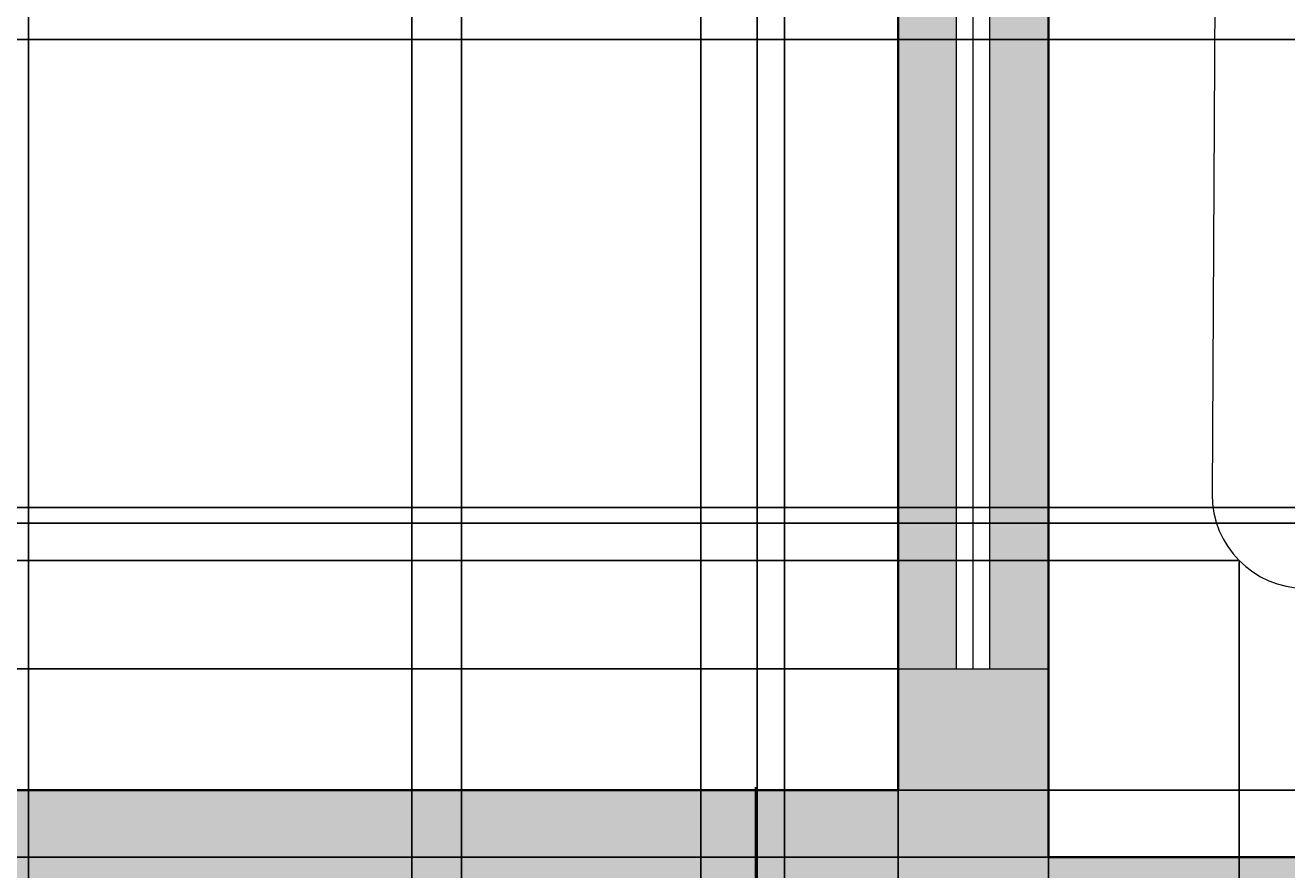
# Model space of a CAD drawing. Units: inches. Extents: x 818 to 1898, y 976 to 2364.
# Tile 29 of 96: x 1207 to 1282, y 1695 to 1746. Entities that reach past the tile are written whole.
import ezdxf

# ---------------------------------------------------------------- set-up
doc = ezdxf.new("R2010")
doc.units = ezdxf.units.IN
doc.header["$LTSCALE"] = 5
doc.header["$MEASUREMENT"] = 0
for name, color, linetype, lineweight in [('A-ANNO-DIMS', 2, 'Continuous', 18), ('A-FURN', 8, 'Continuous', 18), ('A-GLAZ', 4, 'Continuous', 18), ('A-WALL', 7, 'Continuous', 40)]:
    doc.layers.add(name, color=color, linetype=linetype, lineweight=lineweight)
doc.layers.add('A-GLAZ-PATT', color=141, linetype='Continuous', lineweight=9, true_color=0xadddf7)
doc.layers.add('A-WALL-PATT', color=251, linetype='Continuous', lineweight=13, true_color=0x636466)
doc.styles.get("Standard").update_dxf_attribs({"font": 'arial.ttf'})
doc.dimstyles.get("Standard").update_dxf_attribs({"dimtxt": 0.18, "dimasz": 0.18, "dimexe": 0.18, "dimexo": 0.0625, "dimgap": 0.09, "dimtad": 0, "dimtih": 1, "dimtoh": 1, "dimdec": 4, "dimzin": 0, "dimdsep": 46, "dimtxsty": 'Standard', "dimcen": 0.09, "dimadec": 0, "dimazin": 0, "dimtfac": 1, "dimtdec": 4, "dimtofl": 0, "dimtmove": 0, "dimatfit": 3, "dimfxl": 1, "dimtolj": 1, "dimtzin": 0, "dimarcsym": 0})

# ---------------------------------------------------------------- blocks, each defined once
blk = doc.blocks.new('SOFA-3-SEAT')
blk.add_line((39.87, 35.861), (5.697, 36.046))
blk.add_arc((5.667, 30.46), 5.586, 89.68982, 179.68982)
blk = doc.blocks.new('*D42')
at = {"layer": 'A-ANNO-DIMS', "color": 0, "lineweight": -2, "ltscale": 5, "transparency": 16777216}
for p, q in [((1250.195, 1683.07), (1250.195, 1700.259)), ((1250.375, 1700.079), (1306.123, 1700.079)), ((1363.82, 1700.079), (1308.072, 1700.079)), ((1364, 1683.07), (1364, 1700.259))]:
    blk.add_line(p, q, dxfattribs=at)
at = {"layer": 'A-ANNO-DIMS', "color": 0, "ltscale": 5, "transparency": 16777216}
for points in [[(1250.375, 1700.109), (1250.375, 1700.049), (1250.195, 1700.079)], [(1363.82, 1700.109), (1363.82, 1700.049), (1364, 1700.079)]]:
    blk.add_solid(points, dxfattribs=at)
at = {"layer": 'Defpoints', "color": 0, "ltscale": 5, "transparency": 16777216}
for p in [(1364, 1700.079), (1250.195, 1683.008), (1364, 1683.008)]:
    blk.add_point(p, dxfattribs=at)
at = {"layer": 'A-ANNO-DIMS', "color": 0, "ltscale": 5, "transparency": 16777216, "insert": (1307.097, 1700.079), "char_height": 0.18, "attachment_point": 5}
blk.add_mtext('\\A1;SOFA 114 TYP.', dxfattribs=at)
blk = doc.blocks.new('*D59')
at = {"layer": 'A-ANNO-DIMS', "color": 0, "lineweight": -2, "ltscale": 5, "transparency": 16777216}
for p, q in [((1251.643, 2300.393), (818.026, 2300.393)), ((818.206, 2300.213), (818.206, 1669.95)), ((818.206, 1039.323), (818.206, 1669.586)), ((896.051, 1039.143), (818.026, 1039.143))]:
    blk.add_line(p, q, dxfattribs=at)
at = {"layer": 'A-ANNO-DIMS', "color": 0, "ltscale": 5, "transparency": 16777216}
for points in [[(818.176, 2300.213), (818.236, 2300.213), (818.206, 2300.393)], [(818.176, 1039.323), (818.236, 1039.323), (818.206, 1039.143)]]:
    blk.add_solid(points, dxfattribs=at)
at = {"layer": 'Defpoints', "color": 0, "ltscale": 5, "transparency": 16777216}
for p in [(818.206, 2300.393), (1251.706, 2300.393), (896.114, 1039.143)]:
    blk.add_point(p, dxfattribs=at)
at = {"layer": 'A-ANNO-DIMS', "color": 0, "ltscale": 5, "transparency": 16777216, "insert": (818.206, 1669.768), "char_height": 0.18, "attachment_point": 5}
blk.add_mtext('\\A1;1261.2', dxfattribs=at)
blk = doc.blocks.new('*D61')
at = {"layer": 'A-ANNO-DIMS', "color": 0, "lineweight": -2, "ltscale": 5, "transparency": 16777216}
for p, q in [((1071.725, 1203.027), (1071.725, 2363.873)), ((1430.725, 1203.027), (1430.725, 2363.873)), ((1071.905, 2363.693), (1250.936, 2363.693)), ((1430.545, 2363.693), (1251.514, 2363.693))]:
    blk.add_line(p, q, dxfattribs=at)
at = {"layer": 'A-ANNO-DIMS', "color": 0, "ltscale": 5, "transparency": 16777216}
for points in [[(1071.905, 2363.723), (1071.905, 2363.663), (1071.725, 2363.693)], [(1430.545, 2363.723), (1430.545, 2363.663), (1430.725, 2363.693)]]:
    blk.add_solid(points, dxfattribs=at)
at = {"layer": 'Defpoints', "color": 0, "ltscale": 5, "transparency": 16777216}
for p in [(1430.725, 2363.693), (1071.725, 1202.964), (1430.725, 1202.964)]:
    blk.add_point(p, dxfattribs=at)
at = {"layer": 'A-ANNO-DIMS', "color": 0, "ltscale": 5, "transparency": 16777216, "insert": (1251.225, 2363.693), "char_height": 0.18, "attachment_point": 5}
blk.add_mtext('\\A1;359', dxfattribs=at)
blk = doc.blocks.new('*D64')
at = {"layer": 'A-ANNO-DIMS', "color": 0, "lineweight": -2, "ltscale": 5, "transparency": 16777216}
for p, q in [((1197.725, 1501.141), (1197.725, 2363.873)), ((1430.725, 1501.141), (1430.725, 2363.873)), ((1197.905, 2363.693), (1313.935, 2363.693)), ((1430.545, 2363.693), (1314.516, 2363.693))]:
    blk.add_line(p, q, dxfattribs=at)
at = {"layer": 'A-ANNO-DIMS', "color": 0, "ltscale": 5, "transparency": 16777216}
for points in [[(1197.905, 2363.723), (1197.905, 2363.663), (1197.725, 2363.693)], [(1430.545, 2363.723), (1430.545, 2363.663), (1430.725, 2363.693)]]:
    blk.add_solid(points, dxfattribs=at)
at = {"layer": 'Defpoints', "color": 0, "ltscale": 5, "transparency": 16777216}
for p in [(1430.725, 2363.693), (1197.725, 1501.078), (1430.725, 1501.078)]:
    blk.add_point(p, dxfattribs=at)
at = {"layer": 'A-ANNO-DIMS', "color": 0, "ltscale": 5, "transparency": 16777216, "insert": (1314.225, 2363.693), "char_height": 0.18, "attachment_point": 5}
blk.add_mtext('\\A1;233', dxfattribs=at)
blk = doc.blocks.new('*D83')
at = {"layer": 'A-ANNO-DIMS', "color": 0, "lineweight": -2, "ltscale": 5, "transparency": 16777216}
for p, q in [((1197.725, 1700.141), (1197.725, 2363.873)), ((1258.725, 1700.141), (1258.725, 2363.873)), ((1197.905, 2363.693), (1228.023, 2363.693)), ((1258.545, 2363.693), (1228.427, 2363.693))]:
    blk.add_line(p, q, dxfattribs=at)
at = {"layer": 'A-ANNO-DIMS', "color": 0, "ltscale": 5, "transparency": 16777216}
for points in [[(1197.905, 2363.723), (1197.905, 2363.663), (1197.725, 2363.693)], [(1258.545, 2363.723), (1258.545, 2363.663), (1258.725, 2363.693)]]:
    blk.add_solid(points, dxfattribs=at)
at = {"layer": 'Defpoints', "color": 0, "ltscale": 5, "transparency": 16777216}
for p in [(1258.725, 2363.693), (1197.725, 1700.078), (1258.725, 1700.078)]:
    blk.add_point(p, dxfattribs=at)
at = {"layer": 'A-ANNO-DIMS', "color": 0, "ltscale": 5, "transparency": 16777216, "insert": (1228.225, 2363.693), "char_height": 0.18, "attachment_point": 5}
blk.add_mtext('\\A1;61', dxfattribs=at)
blk = doc.blocks.new('*D85')
at = {"layer": 'A-ANNO-DIMS', "color": 0, "lineweight": -2, "ltscale": 5, "transparency": 16777216}
for p, q in [((1258.788, 2053.078), (1897.916, 2053.078)), ((1897.736, 2052.898), (1897.736, 1876.76)), ((1897.736, 1700.258), (1897.736, 1876.396)), ((1258.788, 1700.078), (1897.916, 1700.078))]:
    blk.add_line(p, q, dxfattribs=at)
at = {"layer": 'A-ANNO-DIMS', "color": 0, "ltscale": 5, "transparency": 16777216}
for points in [[(1897.706, 2052.898), (1897.766, 2052.898), (1897.736, 2053.078)], [(1897.706, 1700.258), (1897.766, 1700.258), (1897.736, 1700.078)]]:
    blk.add_solid(points, dxfattribs=at)
at = {"layer": 'Defpoints', "color": 0, "ltscale": 5, "transparency": 16777216}
for p in [(1258.725, 2053.078), (1897.736, 2053.078), (1258.725, 1700.078)]:
    blk.add_point(p, dxfattribs=at)
at = {"layer": 'A-ANNO-DIMS', "color": 0, "ltscale": 5, "transparency": 16777216, "insert": (1897.736, 1876.578), "char_height": 0.18, "attachment_point": 5}
blk.add_mtext('\\A1;353', dxfattribs=at)
blk = doc.blocks.new('*D95')
at = {"layer": 'A-ANNO-DIMS', "color": 0, "lineweight": -2, "ltscale": 5, "transparency": 16777216}
for p, q in [((1173.542, 1071.118), (1173.542, 2363.873)), ((1229.647, 1071.118), (1229.647, 2363.873)), ((1173.722, 2363.693), (1201.288, 2363.693)), ((1229.467, 2363.693), (1201.901, 2363.693))]:
    blk.add_line(p, q, dxfattribs=at)
at = {"layer": 'A-ANNO-DIMS', "color": 0, "ltscale": 5, "transparency": 16777216}
for points in [[(1173.722, 2363.723), (1173.722, 2363.663), (1173.542, 2363.693)], [(1229.467, 2363.723), (1229.467, 2363.663), (1229.647, 2363.693)]]:
    blk.add_solid(points, dxfattribs=at)
at = {"layer": 'Defpoints', "color": 0, "ltscale": 5, "transparency": 16777216}
for p in [(1229.647, 2363.693), (1173.542, 1071.055), (1229.647, 1071.055)]:
    blk.add_point(p, dxfattribs=at)
at = {"layer": 'A-ANNO-DIMS', "color": 0, "ltscale": 5, "transparency": 16777216, "insert": (1201.595, 2363.693), "char_height": 0.18, "attachment_point": 5}
blk.add_mtext('\\A1;56.1', dxfattribs=at)
blk = doc.blocks.new('*D96')
at = {"layer": 'A-ANNO-DIMS', "color": 0, "lineweight": -2, "ltscale": 5, "transparency": 16777216}
for p, q in [((1229.647, 1071.118), (1229.647, 2363.873)), ((1284.17, 1071.118), (1284.17, 2363.873)), ((1229.827, 2363.693), (1256.516, 2363.693)), ((1283.99, 2363.693), (1257.301, 2363.693))]:
    blk.add_line(p, q, dxfattribs=at)
at = {"layer": 'A-ANNO-DIMS', "color": 0, "ltscale": 5, "transparency": 16777216}
for points in [[(1229.827, 2363.723), (1229.827, 2363.663), (1229.647, 2363.693)], [(1283.99, 2363.723), (1283.99, 2363.663), (1284.17, 2363.693)]]:
    blk.add_solid(points, dxfattribs=at)
at = {"layer": 'Defpoints', "color": 0, "ltscale": 5, "transparency": 16777216}
for p in [(1284.17, 2363.693), (1229.647, 1071.055), (1284.17, 1071.055)]:
    blk.add_point(p, dxfattribs=at)
at = {"layer": 'A-ANNO-DIMS', "color": 0, "ltscale": 5, "transparency": 16777216, "insert": (1256.909, 2363.693), "char_height": 0.18, "attachment_point": 5}
blk.add_mtext('\\A1;54.52', dxfattribs=at)
blk = doc.blocks.new('*D119')
at = {"layer": 'A-ANNO-DIMS', "color": 0, "lineweight": -2, "ltscale": 5, "transparency": 16777216}
for p, q in [((1766.29, 1716.987), (818.026, 1716.987)), ((818.206, 1716.807), (818.206, 1672.428)), ((818.206, 1627.685), (818.206, 1672.064)), ((1766.29, 1627.505), (818.026, 1627.505))]:
    blk.add_line(p, q, dxfattribs=at)
at = {"layer": 'A-ANNO-DIMS', "color": 0, "ltscale": 5, "transparency": 16777216}
for points in [[(818.176, 1716.807), (818.236, 1716.807), (818.206, 1716.987)], [(818.176, 1627.685), (818.236, 1627.685), (818.206, 1627.505)]]:
    blk.add_solid(points, dxfattribs=at)
at = {"layer": 'Defpoints', "color": 0, "ltscale": 5, "transparency": 16777216}
for p in [(818.206, 1716.987), (1766.352, 1716.987), (1766.352, 1627.505)]:
    blk.add_point(p, dxfattribs=at)
at = {"layer": 'A-ANNO-DIMS', "color": 0, "ltscale": 5, "transparency": 16777216, "insert": (818.206, 1672.246), "char_height": 0.18, "attachment_point": 5}
blk.add_mtext('\\A1;89.48', dxfattribs=at)
blk = doc.blocks.new('*D120')
at = {"layer": 'A-ANNO-DIMS', "color": 0, "lineweight": -2, "ltscale": 5, "transparency": 16777216}
for p, q in [((1766.29, 1797.717), (818.026, 1797.717)), ((818.206, 1797.537), (818.206, 1757.534)), ((818.206, 1717.167), (818.206, 1757.17)), ((1766.29, 1716.987), (818.026, 1716.987))]:
    blk.add_line(p, q, dxfattribs=at)
at = {"layer": 'A-ANNO-DIMS', "color": 0, "ltscale": 5, "transparency": 16777216}
for points in [[(818.176, 1797.537), (818.236, 1797.537), (818.206, 1797.717)], [(818.176, 1717.167), (818.236, 1717.167), (818.206, 1716.987)]]:
    blk.add_solid(points, dxfattribs=at)
at = {"layer": 'Defpoints', "color": 0, "ltscale": 5, "transparency": 16777216}
for p in [(818.206, 1797.717), (1766.352, 1797.717), (1766.352, 1716.987)]:
    blk.add_point(p, dxfattribs=at)
at = {"layer": 'A-ANNO-DIMS', "color": 0, "ltscale": 5, "transparency": 16777216, "insert": (818.206, 1757.352), "char_height": 0.18, "attachment_point": 5}
blk.add_mtext('\\A1;80.73', dxfattribs=at)
blk = doc.blocks.new('*D145')
at = {"layer": 'A-ANNO-DIMS', "color": 0, "lineweight": -2, "ltscale": 5, "transparency": 16777216}
for p, q in [((1197.393, 2122.314), (1197.393, 975.663)), ((1232.609, 2122.314), (1232.609, 975.663)), ((1197.573, 975.843), (1214.608, 975.843)), ((1232.429, 975.843), (1215.394, 975.843))]:
    blk.add_line(p, q, dxfattribs=at)
at = {"layer": 'A-ANNO-DIMS', "color": 0, "ltscale": 5, "transparency": 16777216}
for points in [[(1197.573, 975.873), (1197.573, 975.813), (1197.393, 975.843)], [(1232.429, 975.873), (1232.429, 975.813), (1232.609, 975.843)]]:
    blk.add_solid(points, dxfattribs=at)
at = {"layer": 'Defpoints', "color": 0, "ltscale": 5, "transparency": 16777216}
for p in [(1197.393, 2122.377), (1232.609, 2122.377), (1232.609, 975.843)]:
    blk.add_point(p, dxfattribs=at)
at = {"layer": 'A-ANNO-DIMS', "color": 0, "ltscale": 5, "transparency": 16777216, "insert": (1215.001, 975.843), "char_height": 0.18, "attachment_point": 5}
blk.add_mtext('\\A1;35.22', dxfattribs=at)
blk = doc.blocks.new('*D215')
at = {"layer": 'A-ANNO-DIMS', "color": 0, "lineweight": -2, "ltscale": 5, "transparency": 16777216}
for p, q in [((1590.663, 1876.078), (818.026, 1876.078)), ((818.206, 1875.898), (818.206, 1781.76)), ((818.206, 1687.258), (818.206, 1781.396)), ((1511.663, 1687.078), (818.026, 1687.078))]:
    blk.add_line(p, q, dxfattribs=at)
at = {"layer": 'A-ANNO-DIMS', "color": 0, "ltscale": 5, "transparency": 16777216}
for points in [[(818.176, 1875.898), (818.236, 1875.898), (818.206, 1876.078)], [(818.176, 1687.258), (818.236, 1687.258), (818.206, 1687.078)]]:
    blk.add_solid(points, dxfattribs=at)
at = {"layer": 'Defpoints', "color": 0, "ltscale": 5, "transparency": 16777216}
for p in [(818.206, 1876.078), (1590.725, 1876.078), (1511.725, 1687.078)]:
    blk.add_point(p, dxfattribs=at)
at = {"layer": 'A-ANNO-DIMS', "color": 0, "ltscale": 5, "transparency": 16777216, "insert": (818.206, 1781.578), "char_height": 0.18, "attachment_point": 5}
blk.add_mtext('\\A1;189', dxfattribs=at)
blk = doc.blocks.new('*D222')
at = {"layer": 'A-ANNO-DIMS', "color": 0, "lineweight": -2, "ltscale": 5, "transparency": 16777216}
for p, q in [((1511.663, 1744.971), (818.026, 1744.971)), ((818.206, 1744.791), (818.206, 1730.69)), ((818.206, 1716.225), (818.206, 1730.327)), ((1511.663, 1716.045), (818.026, 1716.045))]:
    blk.add_line(p, q, dxfattribs=at)
at = {"layer": 'A-ANNO-DIMS', "color": 0, "ltscale": 5, "transparency": 16777216}
for points in [[(818.176, 1744.791), (818.236, 1744.791), (818.206, 1744.971)], [(818.176, 1716.225), (818.236, 1716.225), (818.206, 1716.045)]]:
    blk.add_solid(points, dxfattribs=at)
at = {"layer": 'Defpoints', "color": 0, "ltscale": 5, "transparency": 16777216}
for p in [(818.206, 1744.971), (1511.725, 1744.971), (1511.725, 1716.045)]:
    blk.add_point(p, dxfattribs=at)
at = {"layer": 'A-ANNO-DIMS', "color": 0, "ltscale": 5, "transparency": 16777216, "insert": (818.206, 1730.508), "char_height": 0.18, "attachment_point": 5}
blk.add_mtext('\\A1;28.926', dxfattribs=at)
blk = doc.blocks.new('*D223')
at = {"layer": 'A-ANNO-DIMS', "color": 0, "lineweight": -2, "ltscale": 5, "transparency": 16777216}
for p, q in [((1511.663, 1716.045), (818.026, 1716.045)), ((818.206, 1715.865), (818.206, 1706.244)), ((818.206, 1696.258), (818.206, 1705.88)), ((1511.663, 1696.078), (818.026, 1696.078))]:
    blk.add_line(p, q, dxfattribs=at)
at = {"layer": 'A-ANNO-DIMS', "color": 0, "ltscale": 5, "transparency": 16777216}
for points in [[(818.176, 1715.865), (818.236, 1715.865), (818.206, 1716.045)], [(818.176, 1696.258), (818.236, 1696.258), (818.206, 1696.078)]]:
    blk.add_solid(points, dxfattribs=at)
at = {"layer": 'Defpoints', "color": 0, "ltscale": 5, "transparency": 16777216}
for p in [(818.206, 1716.045), (1511.725, 1716.045), (1511.725, 1696.078)]:
    blk.add_point(p, dxfattribs=at)
at = {"layer": 'A-ANNO-DIMS', "color": 0, "ltscale": 5, "transparency": 16777216, "insert": (818.206, 1706.062), "char_height": 0.18, "attachment_point": 5}
blk.add_mtext('\\A1;19.967', dxfattribs=at)
blk = doc.blocks.new('*D233')
at = {"layer": 'A-ANNO-DIMS', "color": 0, "lineweight": -2, "ltscale": 5, "transparency": 16777216}
for p, q in [((1267.725, 2044.016), (1267.725, 975.663)), ((1303.931, 2008.329), (1303.931, 975.663)), ((1267.905, 975.843), (1285.365, 975.843)), ((1303.751, 975.843), (1286.292, 975.843))]:
    blk.add_line(p, q, dxfattribs=at)
at = {"layer": 'A-ANNO-DIMS', "color": 0, "ltscale": 5, "transparency": 16777216}
for points in [[(1267.905, 975.873), (1267.905, 975.813), (1267.725, 975.843)], [(1303.751, 975.873), (1303.751, 975.813), (1303.931, 975.843)]]:
    blk.add_solid(points, dxfattribs=at)
at = {"layer": 'Defpoints', "color": 0, "ltscale": 5, "transparency": 16777216}
for p in [(1267.725, 2044.078), (1303.931, 2008.392), (1303.931, 975.843)]:
    blk.add_point(p, dxfattribs=at)
at = {"layer": 'A-ANNO-DIMS', "color": 0, "ltscale": 5, "transparency": 16777216, "insert": (1285.828, 975.843), "char_height": 0.18, "attachment_point": 5}
blk.add_mtext('\\A1;36.206', dxfattribs=at)
blk = doc.blocks.new('*D246')
at = {"layer": 'A-ANNO-DIMS', "color": 0, "lineweight": -2, "ltscale": 5, "transparency": 16777216}
for p, q in [((1258.663, 1755.332), (818.026, 1755.332)), ((818.206, 1755.152), (818.206, 1731.514)), ((818.206, 1707.512), (818.206, 1731.15)), ((1258.663, 1707.332), (818.026, 1707.332))]:
    blk.add_line(p, q, dxfattribs=at)
at = {"layer": 'A-ANNO-DIMS', "color": 0, "ltscale": 5, "transparency": 16777216}
for points in [[(818.176, 1755.152), (818.236, 1755.152), (818.206, 1755.332)], [(818.176, 1707.512), (818.236, 1707.512), (818.206, 1707.332)]]:
    blk.add_solid(points, dxfattribs=at)
at = {"layer": 'Defpoints', "color": 0, "ltscale": 5, "transparency": 16777216}
for p in [(818.206, 1755.332), (1258.725, 1755.332), (1258.725, 1707.332)]:
    blk.add_point(p, dxfattribs=at)
at = {"layer": 'A-ANNO-DIMS', "color": 0, "ltscale": 5, "transparency": 16777216, "insert": (818.206, 1731.332), "char_height": 0.18, "attachment_point": 5}
blk.add_mtext('\\A1;48', dxfattribs=at)
blk = doc.blocks.new('*D251')
at = {"layer": 'A-ANNO-DIMS', "color": 0, "lineweight": -2, "ltscale": 5, "transparency": 16777216}
for p, q in [((1250.303, 1878.329), (1250.303, 975.663)), ((1258.725, 1878.329), (1258.725, 975.663)), ((1250.483, 975.843), (1254.121, 975.843)), ((1258.545, 975.843), (1254.907, 975.843))]:
    blk.add_line(p, q, dxfattribs=at)
at = {"layer": 'A-ANNO-DIMS', "color": 0, "ltscale": 5, "transparency": 16777216}
for points in [[(1250.483, 975.873), (1250.483, 975.813), (1250.303, 975.843)], [(1258.545, 975.873), (1258.545, 975.813), (1258.725, 975.843)]]:
    blk.add_solid(points, dxfattribs=at)
at = {"layer": 'Defpoints', "color": 0, "ltscale": 5, "transparency": 16777216}
for p in [(1250.303, 1878.392), (1258.725, 1878.392), (1258.725, 975.843)]:
    blk.add_point(p, dxfattribs=at)
at = {"layer": 'A-ANNO-DIMS', "color": 0, "ltscale": 5, "transparency": 16777216, "insert": (1254.514, 975.843), "char_height": 0.18, "attachment_point": 5}
blk.add_mtext('\\A1;8.422', dxfattribs=at)
blk = doc.blocks.new('*D254')
at = {"layer": 'A-ANNO-DIMS', "color": 0, "lineweight": -2, "ltscale": 5, "transparency": 16777216}
for p, q in [((1267.725, 2044.016), (1267.725, 975.663)), ((1330.305, 2044.016), (1330.305, 975.663)), ((1267.905, 975.843), (1298.621, 975.843)), ((1330.125, 975.843), (1299.409, 975.843))]:
    blk.add_line(p, q, dxfattribs=at)
at = {"layer": 'A-ANNO-DIMS', "color": 0, "ltscale": 5, "transparency": 16777216}
for points in [[(1267.905, 975.873), (1267.905, 975.813), (1267.725, 975.843)], [(1330.125, 975.873), (1330.125, 975.813), (1330.305, 975.843)]]:
    blk.add_solid(points, dxfattribs=at)
at = {"layer": 'Defpoints', "color": 0, "ltscale": 5, "transparency": 16777216}
for p in [(1267.725, 2044.078), (1330.305, 2044.078), (1330.305, 975.843)]:
    blk.add_point(p, dxfattribs=at)
at = {"layer": 'A-ANNO-DIMS', "color": 0, "ltscale": 5, "transparency": 16777216, "insert": (1299.015, 975.843), "char_height": 0.18, "attachment_point": 5}
blk.add_mtext('\\A1;62.58', dxfattribs=at)
blk = doc.blocks.new('*D269')
at = {"layer": 'A-ANNO-DIMS', "color": 0, "lineweight": -2, "ltscale": 5, "transparency": 16777216}
for p, q in [((1246.938, 1534.141), (1246.938, 2363.873)), ((1341.259, 1534.141), (1341.259, 2363.873)), ((1247.118, 2363.693), (1293.706, 2363.693)), ((1341.079, 2363.693), (1294.491, 2363.693))]:
    blk.add_line(p, q, dxfattribs=at)
at = {"layer": 'A-ANNO-DIMS', "color": 0, "ltscale": 5, "transparency": 16777216}
for points in [[(1247.118, 2363.723), (1247.118, 2363.663), (1246.938, 2363.693)], [(1341.079, 2363.723), (1341.079, 2363.663), (1341.259, 2363.693)]]:
    blk.add_solid(points, dxfattribs=at)
at = {"layer": 'Defpoints', "color": 0, "ltscale": 5, "transparency": 16777216}
for p in [(1341.259, 2363.693), (1246.938, 1534.078), (1341.259, 1534.078)]:
    blk.add_point(p, dxfattribs=at)
at = {"layer": 'A-ANNO-DIMS', "color": 0, "ltscale": 5, "transparency": 16777216, "insert": (1294.099, 2363.693), "char_height": 0.18, "attachment_point": 5}
blk.add_mtext('\\A1;94.32', dxfattribs=at)
blk = doc.blocks.new('*D271')
at = {"layer": 'A-ANNO-DIMS', "color": 0, "lineweight": -2, "ltscale": 5, "transparency": 16777216}
for p, q in [((1206.725, 1510.141), (1206.725, 2363.873)), ((1246.938, 1510.141), (1246.938, 2363.873)), ((1206.905, 2363.693), (1226.451, 2363.693)), ((1246.758, 2363.693), (1227.211, 2363.693))]:
    blk.add_line(p, q, dxfattribs=at)
at = {"layer": 'A-ANNO-DIMS', "color": 0, "ltscale": 5, "transparency": 16777216}
for points in [[(1206.905, 2363.723), (1206.905, 2363.663), (1206.725, 2363.693)], [(1246.758, 2363.723), (1246.758, 2363.663), (1246.938, 2363.693)]]:
    blk.add_solid(points, dxfattribs=at)
at = {"layer": 'Defpoints', "color": 0, "ltscale": 5, "transparency": 16777216}
for p in [(1246.938, 2363.693), (1206.725, 1510.078), (1246.938, 1510.078)]:
    blk.add_point(p, dxfattribs=at)
at = {"layer": 'A-ANNO-DIMS', "color": 0, "ltscale": 5, "transparency": 16777216, "insert": (1226.831, 2363.693), "char_height": 0.18, "attachment_point": 5}
blk.add_mtext('\\A1;40.21', dxfattribs=at)
blk = doc.blocks.new('*D276')
at = {"layer": 'A-ANNO-DIMS', "color": 0, "lineweight": -2, "ltscale": 5, "transparency": 16777216}
for p, q in [((1206.725, 1687.141), (1206.725, 2363.873)), ((1251.933, 1681.439), (1251.933, 2363.873)), ((1206.905, 2363.693), (1228.949, 2363.693)), ((1251.753, 2363.693), (1229.709, 2363.693))]:
    blk.add_line(p, q, dxfattribs=at)
at = {"layer": 'A-ANNO-DIMS', "color": 0, "ltscale": 5, "transparency": 16777216}
for points in [[(1206.905, 2363.723), (1206.905, 2363.663), (1206.725, 2363.693)], [(1251.753, 2363.723), (1251.753, 2363.663), (1251.933, 2363.693)]]:
    blk.add_solid(points, dxfattribs=at)
at = {"layer": 'Defpoints', "color": 0, "ltscale": 5, "transparency": 16777216}
for p in [(1251.933, 2363.693), (1206.725, 1687.078), (1251.933, 1681.376)]:
    blk.add_point(p, dxfattribs=at)
at = {"layer": 'A-ANNO-DIMS', "color": 0, "ltscale": 5, "transparency": 16777216, "insert": (1229.329, 2363.693), "char_height": 0.18, "attachment_point": 5}
blk.add_mtext('\\A1;45.21', dxfattribs=at)
blk = doc.blocks.new('*D278')
at = {"layer": 'A-ANNO-DIMS', "color": 0, "lineweight": -2, "ltscale": 5, "transparency": 16777216}
for p, q in [((1324.033, 1700.743), (1324.033, 975.663)), ((1267.725, 1696.016), (1267.725, 975.663)), ((1267.905, 975.843), (1295.503, 975.843)), ((1323.853, 975.843), (1296.256, 975.843))]:
    blk.add_line(p, q, dxfattribs=at)
at = {"layer": 'A-ANNO-DIMS', "color": 0, "ltscale": 5, "transparency": 16777216}
for points in [[(1267.905, 975.873), (1267.905, 975.813), (1267.725, 975.843)], [(1323.853, 975.873), (1323.853, 975.813), (1324.033, 975.843)]]:
    blk.add_solid(points, dxfattribs=at)
at = {"layer": 'Defpoints', "color": 0, "ltscale": 5, "transparency": 16777216}
for p in [(1324.033, 1700.806), (1267.725, 1696.078), (1324.033, 975.843)]:
    blk.add_point(p, dxfattribs=at)
at = {"layer": 'A-ANNO-DIMS', "color": 0, "ltscale": 5, "transparency": 16777216, "insert": (1295.879, 975.843), "char_height": 0.18, "attachment_point": 5}
blk.add_mtext('\\A1;56.31', dxfattribs=at)
blk = doc.blocks.new('*D279')
at = {"layer": 'A-ANNO-DIMS', "color": 0, "lineweight": -2, "ltscale": 5, "transparency": 16777216}
for p, q in [((1279.125, 1713.755), (1279.125, 975.663)), ((1267.725, 1696.016), (1267.725, 975.663)), ((1267.905, 975.843), (1273.11, 975.843)), ((1278.945, 975.843), (1273.74, 975.843))]:
    blk.add_line(p, q, dxfattribs=at)
at = {"layer": 'A-ANNO-DIMS', "color": 0, "ltscale": 5, "transparency": 16777216}
for points in [[(1267.905, 975.873), (1267.905, 975.813), (1267.725, 975.843)], [(1278.945, 975.873), (1278.945, 975.813), (1279.125, 975.843)]]:
    blk.add_solid(points, dxfattribs=at)
at = {"layer": 'Defpoints', "color": 0, "ltscale": 5, "transparency": 16777216}
for p in [(1279.125, 1713.817), (1267.725, 1696.078), (1267.725, 975.843)]:
    blk.add_point(p, dxfattribs=at)
at = {"layer": 'A-ANNO-DIMS', "color": 0, "ltscale": 5, "transparency": 16777216, "insert": (1273.425, 975.843), "char_height": 0.18, "attachment_point": 5}
blk.add_mtext('\\A1;11.4', dxfattribs=at)
blk = doc.blocks.new('*D283')
at = {"layer": 'A-ANNO-DIMS', "color": 0, "lineweight": -2, "ltscale": 5, "transparency": 16777216}
for p, q in [((1351.599, 1761.386), (1351.599, 975.663)), ((1267.725, 1696.016), (1267.725, 975.663)), ((1267.905, 975.843), (1309.268, 975.843)), ((1351.419, 975.843), (1310.056, 975.843))]:
    blk.add_line(p, q, dxfattribs=at)
at = {"layer": 'A-ANNO-DIMS', "color": 0, "ltscale": 5, "transparency": 16777216}
for points in [[(1267.905, 975.873), (1267.905, 975.813), (1267.725, 975.843)], [(1351.419, 975.873), (1351.419, 975.813), (1351.599, 975.843)]]:
    blk.add_solid(points, dxfattribs=at)
at = {"layer": 'Defpoints', "color": 0, "ltscale": 5, "transparency": 16777216}
for p in [(1351.599, 1761.449), (1267.725, 1696.078), (1351.599, 975.843)]:
    blk.add_point(p, dxfattribs=at)
at = {"layer": 'A-ANNO-DIMS', "color": 0, "ltscale": 5, "transparency": 16777216, "insert": (1309.662, 975.843), "char_height": 0.18, "attachment_point": 5}
blk.add_mtext('\\A1;83.87', dxfattribs=at)
blk = doc.blocks.new('*D284')
at = {"layer": 'A-ANNO-DIMS', "color": 0, "lineweight": -2, "ltscale": 5, "transparency": 16777216}
for p, q in [((1351.661, 1761.449), (1897.916, 1761.449)), ((1897.736, 1761.269), (1897.736, 1728.946)), ((1897.736, 1696.258), (1897.736, 1728.582)), ((1267.788, 1696.078), (1897.916, 1696.078))]:
    blk.add_line(p, q, dxfattribs=at)
at = {"layer": 'A-ANNO-DIMS', "color": 0, "ltscale": 5, "transparency": 16777216}
for points in [[(1897.706, 1761.269), (1897.766, 1761.269), (1897.736, 1761.449)], [(1897.706, 1696.258), (1897.766, 1696.258), (1897.736, 1696.078)]]:
    blk.add_solid(points, dxfattribs=at)
at = {"layer": 'Defpoints', "color": 0, "ltscale": 5, "transparency": 16777216}
for p in [(1351.599, 1761.449), (1267.725, 1696.078), (1897.736, 1696.078)]:
    blk.add_point(p, dxfattribs=at)
at = {"layer": 'A-ANNO-DIMS', "color": 0, "ltscale": 5, "transparency": 16777216, "insert": (1897.736, 1728.764), "char_height": 0.18, "attachment_point": 5}
blk.add_mtext('\\A1;65.37', dxfattribs=at)
blk = doc.blocks.new('*D285')
at = {"layer": 'A-ANNO-DIMS', "color": 0, "lineweight": -2, "ltscale": 5, "transparency": 16777216}
for p, q in [((1305.828, 1830.022), (1305.828, 975.663)), ((1267.725, 1814.903), (1267.725, 975.663)), ((1267.905, 975.843), (1286.47, 975.843)), ((1305.648, 975.843), (1287.083, 975.843))]:
    blk.add_line(p, q, dxfattribs=at)
at = {"layer": 'A-ANNO-DIMS', "color": 0, "ltscale": 5, "transparency": 16777216}
for points in [[(1267.905, 975.873), (1267.905, 975.813), (1267.725, 975.843)], [(1305.648, 975.873), (1305.648, 975.813), (1305.828, 975.843)]]:
    blk.add_solid(points, dxfattribs=at)
at = {"layer": 'Defpoints', "color": 0, "ltscale": 5, "transparency": 16777216}
for p in [(1305.828, 1830.084), (1267.725, 1814.965), (1267.725, 975.843)]:
    blk.add_point(p, dxfattribs=at)
at = {"layer": 'A-ANNO-DIMS', "color": 0, "ltscale": 5, "transparency": 16777216, "insert": (1286.776, 975.843), "char_height": 0.18, "attachment_point": 5}
blk.add_mtext('\\A1;38.1', dxfattribs=at)
blk = doc.blocks.new('*D289')
at = {"layer": 'A-ANNO-DIMS', "color": 0, "lineweight": -2, "ltscale": 5, "transparency": 16777216}
for p, q in [((1279.063, 1713.817), (818.026, 1713.817)), ((818.206, 1713.637), (818.206, 1705.128)), ((818.206, 1696.258), (818.206, 1704.767)), ((1267.663, 1696.078), (818.026, 1696.078))]:
    blk.add_line(p, q, dxfattribs=at)
at = {"layer": 'A-ANNO-DIMS', "color": 0, "ltscale": 5, "transparency": 16777216}
for points in [[(818.176, 1713.637), (818.236, 1713.637), (818.206, 1713.817)], [(818.176, 1696.258), (818.236, 1696.258), (818.206, 1696.078)]]:
    blk.add_solid(points, dxfattribs=at)
at = {"layer": 'Defpoints', "color": 0, "ltscale": 5, "transparency": 16777216}
for p in [(1279.125, 1713.817), (818.206, 1696.078), (1267.725, 1696.078)]:
    blk.add_point(p, dxfattribs=at)
at = {"layer": 'A-ANNO-DIMS', "color": 0, "ltscale": 5, "transparency": 16777216, "insert": (818.206, 1704.948), "char_height": 0.18, "attachment_point": 5}
blk.add_mtext('\\A1;17.74', dxfattribs=at)

msp = doc.modelspace()

# ---------------------------------------------------------------- hatches: boundary and pattern name
at = {"layer": 'A-GLAZ-PATT', "ltscale": 5}
h = msp.add_hatch(color=256, dxfattribs=at)
h.dxf.hatch_style = 1
h.paths.add_polyline_path([(1283.8183, 1504.5782), (1206.7251, 1504.5782), (1206.7251, 1501.0782), (1283.8183, 1501.0782)])
h.paths.add_polyline_path([(1283.8183, 1510.0782), (1206.7251, 1510.0782), (1206.7251, 1506.5782), (1283.8183, 1506.5782)])
h.paths.add_polyline_path([(1490.9163, 1355.0782), (1439.7252, 1355.0782), (1439.7252, 1409.0522), (1436.2252, 1409.0522), (1436.2252, 1351.5782), (1490.9163, 1351.5782)])
h.paths.add_polyline_path([(1434.2252, 1409.0522), (1430.7251, 1409.0522), (1430.7251, 1346.0782), (1435.0799, 1346.0782), (1435.0731, 1346.1152), (1435.1501, 1346.0782), (1490.9163, 1346.0782), (1490.9163, 1349.5782), (1434.2252, 1349.5782)])
h.paths.add_polyline_path([(1714.7252, 1545.0782), (1711.2252, 1545.0782), (1711.2252, 1521.0782), (1714.7252, 1521.0782)])
h.paths.add_polyline_path([(1709.2252, 1545.0782), (1705.7252, 1545.0782), (1705.7252, 1521.0782), (1709.2252, 1521.0782)])
h.paths.add_polyline_path([(1714.7252, 1687.0782), (1711.2252, 1687.0782), (1711.2252, 1649.9029), (1714.7252, 1649.9029)])
h.paths.add_polyline_path([(1709.2252, 1687.0782), (1705.7252, 1687.0782), (1705.7252, 1649.9029), (1709.2252, 1649.9029)])
h.paths.add_polyline_path([(1709.2252, 1745.5584), (1705.7252, 1745.5584), (1705.7252, 1717.3178), (1709.2252, 1717.3178)])
h.paths.add_polyline_path([(1714.7252, 1745.5584), (1711.2252, 1745.5584), (1711.2252, 1717.3178), (1714.7252, 1717.3178)])
h.paths.add_polyline_path([(1714.7252, 2014.5114), (1711.2252, 2014.5114), (1711.2252, 1962.0338), (1714.7252, 1962.0338)])
h.paths.add_polyline_path([(1709.2252, 2014.5114), (1705.7252, 2014.5114), (1705.7252, 1962.0338), (1709.2252, 1962.0338)])
h.paths.add_polyline_path([(1538.5155, 2047.5782), (1485.1216, 2047.5782), (1485.1216, 2044.0782), (1538.5155, 2044.0782)])
h.paths.add_polyline_path([(1538.5155, 2053.0782), (1485.1216, 2053.0782), (1485.1216, 2049.5782), (1538.5155, 2049.5782)])
h.paths.add_polyline_path([(1388.0315, 2047.5782), (1330.305, 2047.5782), (1330.305, 2044.0782), (1388.0315, 2044.0782)])
h.paths.add_polyline_path([(1388.0315, 2053.0782), (1330.305, 2053.0782), (1330.305, 2049.5782), (1388.0315, 2049.5782)])
h.paths.add_polyline_path([(1262.2252, 2019.2871), (1258.7251, 2019.2871), (1258.7251, 1928.9218), (1262.2252, 1928.9218)])
h.paths.add_polyline_path([(1267.7251, 2019.2871), (1264.2252, 2019.2871), (1264.2252, 1928.9218), (1267.7251, 1928.9218)])
h.paths.add_polyline_path([(1262.2252, 1862.9652), (1258.7251, 1862.9652), (1258.7251, 1814.9652), (1262.2252, 1814.9652)])
h.paths.add_polyline_path([(1267.7251, 1862.9652), (1264.2252, 1862.9652), (1264.2252, 1814.9652), (1267.7251, 1814.9652)])
h.paths.add_polyline_path([(1262.2252, 1755.3321), (1258.7251, 1755.3321), (1258.7251, 1707.3321), (1262.2252, 1707.3321)])
h.paths.add_polyline_path([(1267.7251, 1755.3321), (1264.2252, 1755.3321), (1264.2252, 1707.3321), (1267.7251, 1707.3321)])
h.paths.add_polyline_path([(1251.9333, 1692.5782), (1206.7251, 1692.5782), (1206.7251, 1687.0782), (1251.9333, 1687.0782)])
h.paths.add_polyline_path([(1251.9333, 1700.0782), (1206.7251, 1700.0782), (1206.7251, 1694.5782), (1251.9333, 1694.5782)])
at = {"layer": 'A-WALL-PATT', "ltscale": 5}
h = msp.add_hatch(color=256, dxfattribs=at)
h.dxf.hatch_style = 1
h.paths.add_polyline_path([(1267.7251, 1928.9218), (1258.7251, 1928.9218), (1258.7251, 1913.6401), (1250.3029, 1913.6401), (1250.3029, 1878.3919), (1258.7251, 1878.3919), (1258.7251, 1862.9652), (1267.7251, 1862.9652)])
h.paths.add_polyline_path([(1267.7251, 1814.9652), (1258.7251, 1814.9652), (1258.7251, 1755.3321), (1267.7251, 1755.3321)])
h.paths.add_polyline_path([(1463.7252, 1696.0782), (1267.7251, 1696.0782), (1267.7251, 1707.3321), (1258.7251, 1707.3321), (1258.7251, 1700.0782), (1251.9333, 1700.0782), (1251.9333, 1687.0782), (1463.7252, 1687.0782)])
h.paths.add_polyline_path([(1714.7252, 1717.3178), (1705.7252, 1717.3178), (1705.7252, 1696.0782), (1599.7252, 1696.0782), (1599.7252, 1790.0782), (1705.7252, 1790.0782), (1705.7252, 1785.6125), (1714.7252, 1785.6125), (1714.7252, 1827.2125), (1705.7252, 1827.2125), (1705.7252, 1802.0782), (1599.7252, 1802.0782), (1599.7252, 1867.0782), (1705.7252, 1867.0782), (1705.7252, 1857.2125), (1714.7252, 1857.2125), (1714.7252, 1930.0316), (1741.8409, 1930.0316), (1741.8409, 1935.0316), (1714.7252, 1935.0316), (1714.7252, 1957.0338), (1741.8409, 1957.0338), (1741.8409, 1962.0338), (1714.7252, 1962.0338), (1705.7252, 1962.0338), (1705.7252, 1948.0782), (1599.7252, 1948.0782), (1599.7252, 1981.0782), (1590.7251, 1981.0782), (1590.7251, 1941.0782), (1620.7252, 1941.0782), (1705.7252, 1941.0782), (1705.7252, 1876.0782), (1599.7252, 1876.0782), (1599.7252, 1911.0782), (1590.7251, 1911.0782), (1590.7251, 1876.0782), (1429.2252, 1876.0782), (1429.2252, 1867.0782), (1511.7251, 1867.0782), (1528.593, 1867.0782), (1595.7252, 1867.0782), (1595.7252, 1773.0782), (1520.7252, 1773.0782), (1520.7252, 1837.5823), (1532.593, 1837.5823), (1532.593, 1867.0782), (1528.593, 1867.0782), (1528.593, 1841.5823), (1511.7251, 1841.5823), (1511.7251, 1744.9714), (1520.7252, 1744.9714), (1520.7252, 1761.0782), (1595.7252, 1761.0782), (1595.7252, 1696.0782), (1520.7252, 1696.0782), (1520.7252, 1716.0454), (1511.7251, 1716.0454), (1511.7251, 1696.0782), (1511.7251, 1687.0782), (1714.7252, 1687.0782)])
h.paths.add_polyline_path([(1714.7252, 2053.0782), (1714.7252, 2081.1881), (1709.7252, 2081.1881), (1709.7252, 2053.0782), (1681.6446, 2053.0782), (1681.6446, 2081.1881), (1676.6446, 2081.1881), (1676.6446, 2053.0782), (1538.5155, 2053.0782), (1538.5155, 2044.0782), (1590.7251, 2044.0782), (1590.7251, 2011.0782), (1599.7252, 2011.0782), (1599.7252, 2044.0782), (1705.7252, 2044.0782), (1705.7252, 2014.5114), (1714.7252, 2014.5114)])
h.paths.add_polyline_path([(1485.1216, 2053.0782), (1422.02, 2053.0782), (1422.02, 2081.1881), (1413.02, 2081.1881), (1413.02, 2053.0782), (1399.6356, 2053.0782), (1399.6356, 2081.1881), (1390.6356, 2081.1881), (1390.6356, 2053.0782), (1388.0315, 2053.0782), (1388.0315, 2044.0782), (1416.2743, 2044.0782), (1485.1216, 2044.0782)])
h.paths.add_polyline_path([(1330.305, 2053.0782), (1258.7251, 2053.0782), (1258.7251, 2019.2871), (1267.7251, 2019.2871), (1267.7251, 2044.0782), (1330.305, 2044.0782)])
h.paths.add_polyline_path([(1258.7251, 2053.0782), (1214.6577, 2053.0782), (1214.6577, 2044.0782), (1258.7251, 2044.0782)])
h.paths.add_polyline_path([(1214.6577, 2053.0782), (1180.349, 2053.0782), (1180.349, 2044.0782), (1214.6577, 2044.0782)])
h.paths.add_polyline_path([(1714.7252, 1639.5782), (1741.8409, 1639.5782), (1741.8409, 1643.5782), (1714.7252, 1643.5782), (1714.7252, 1649.9029), (1705.7252, 1649.9029), (1705.7252, 1600.0782), (1477.7252, 1600.0782), (1477.7252, 1591.0782), (1520.7252, 1591.0782), (1616.7252, 1591.0782), (1616.7252, 1416.6857), (1622.7252, 1416.6857), (1622.7252, 1463.0782), (1624.7252, 1463.0782), (1624.7252, 1467.0782), (1622.7252, 1467.0782), (1622.7252, 1591.0782), (1705.7252, 1591.0782), (1705.7252, 1545.0782), (1714.7252, 1545.0782), (1741.8409, 1545.0782), (1741.8409, 1549.0782), (1714.7252, 1549.0782), (1714.7252, 1593.9175), (1737.8409, 1593.9175), (1737.8409, 1597.9175), (1714.7252, 1597.9175)])
h.paths.add_polyline_path([(1674.9024, 2060.7419), (1714.7045, 2060.7419), (1714.7045, 2073.1061), (1674.9024, 2073.1061)], flags=25)
h.paths.add_polyline_path([(1394.5468, 2061.6618), (1422.2344, 2061.6618), (1422.2344, 2074.0261), (1394.5468, 2074.0261)], flags=24)
h = msp.add_hatch(color=256, dxfattribs=at)
h.dxf.hatch_style = 1
h.paths.add_polyline_path([(1206.7251, 1687.0782), (1206.7251, 1700.0782), (1197.7251, 1700.0782), (1197.7251, 1501.0782), (1206.7251, 1501.0782), (1206.7251, 1510.0782)])
h.paths.add_polyline_path([(1197.7251, 1590.7585), (1173.7252, 1590.7585), (1173.7252, 1586.7585), (1197.7251, 1586.7585)])
h.paths.add_polyline_path([(1197.7251, 1534.6024), (1173.7252, 1534.6024), (1173.7252, 1530.6024), (1197.7251, 1530.6024)])
h.paths.add_polyline_path([(1365.1463, 1510.0782), (1283.8183, 1510.0782), (1283.8183, 1501.0782), (1365.1463, 1501.0782)])
h.paths.add_polyline_path([(1439.7252, 1591.0782), (1441.7252, 1591.0782), (1441.7252, 1600.0782), (1430.7251, 1600.0782), (1430.7251, 1510.0782), (1406.7252, 1510.0782), (1401.1463, 1510.0782), (1401.1463, 1501.0782), (1430.7251, 1501.0782), (1430.7251, 1486.2383), (1430.7251, 1409.0522), (1439.7252, 1409.0522)])

# ---------------------------------------------------------------- linework, layer by layer
at = {"layer": 'A-GLAZ'}
for p, q in [((1262.2252, 1707.3321), (1262.2252, 1755.3321)), ((1263.2252, 1707.3321), (1263.2252, 1755.3321)), ((1264.2252, 1707.3321), (1264.2252, 1755.3321)), ((1258.7251, 1707.3321), (1267.7251, 1707.3321)), ((1206.7251, 1687.0782), (1206.7251, 1700.0782)), ((1251.9333, 1700.0782), (1251.9333, 1687.0782))]:
    msp.add_line(p, q, dxfattribs=at)
at = {"layer": 'A-WALL'}
for p, q in [((1258.7251, 1878.3919), (1258.7251, 1700.0782)), ((1267.7251, 1867.0782), (1267.7251, 1696.0782)), ((1197.7251, 1700.0782), (1258.7251, 1700.0782)), ((1267.7251, 1696.0782), (1463.7252, 1696.0782))]:
    msp.add_line(p, q, dxfattribs=at)

# ---------------------------------------------------------------- block references
at = {"layer": 'A-FURN', "rotation": 90.0000000000007}
msp.add_blockref('SOFA-3-SEAT', (1313.5566, 1712.0791), dxfattribs=at)

# ---------------------------------------------------------------- dimensions: what is measured, and where the dimension line sits
at = {"layer": 'A-ANNO-DIMS', "ltscale": 5}
for base, p1, p2, override, picture, middle in [((1430.7251, 2363.6929), (1071.7251, 1202.9642), (1430.7251, 1202.9642), {"dimdec": 0, "dimlfac": 1, "dimrnd": 0, "dimzin": 0, "dimdsep": 46, "dimlunit": 2}, '*D61', (1251.2251, 2363.6929)), ((1229.6474, 2363.6929), (1173.5418, 1071.0552), (1229.6474, 1071.0552), {"dimdec": 1, "dimlfac": 1, "dimrnd": 0, "dimzin": 0, "dimdsep": 46, "dimlunit": 2}, '*D95', (1201.5946, 2363.6929)), ((1430.7251, 2363.6929), (1197.7251, 1501.0782), (1430.7251, 1501.0782), {"dimdec": 0, "dimlfac": 1, "dimrnd": 0, "dimzin": 0, "dimdsep": 46, "dimlunit": 2}, '*D64', (1314.2251, 2363.6929)), ((1258.7251, 2363.6929), (1197.7251, 1700.0782), (1258.7251, 1700.0782), {"dimdec": 0, "dimlfac": 1, "dimrnd": 0, "dimzin": 0, "dimdsep": 46, "dimlunit": 2}, '*D83', (1228.2251, 2363.6929)), ((1246.9377, 2363.6929), (1206.7251, 1510.0782), (1246.9377, 1510.0782), {"dimdec": 2, "dimlfac": 1, "dimrnd": 0, "dimzin": 0, "dimdsep": 46, "dimlunit": 2}, '*D271', (1226.8314, 2363.6929)), ((1251.9333, 2363.6929), (1206.7251, 1687.0782), (1251.9333, 1681.3763), {"dimdec": 2, "dimlfac": 1, "dimrnd": 0, "dimzin": 0, "dimdsep": 46, "dimlunit": 2}, '*D276', (1229.3292, 2363.6929)), ((1284.1697, 2363.6929), (1229.6474, 1071.0552), (1284.1697, 1071.0552), {"dimdec": 2, "dimlfac": 1, "dimrnd": 0, "dimzin": 0, "dimdsep": 46, "dimlunit": 2}, '*D96', (1256.9085, 2363.6929)), ((1341.2593, 2363.6929), (1246.9377, 1534.0782), (1341.2593, 1534.0782), {"dimdec": 2, "dimlfac": 1, "dimrnd": 0, "dimzin": 0, "dimdsep": 46, "dimlunit": 2}, '*D269', (1294.0985, 2363.6929)), ((1232.6091, 975.8433), (1197.3925, 2122.3767), (1232.6091, 2122.3767), {"dimdec": 2, "dimlfac": 1, "dimrnd": 0, "dimzin": 0, "dimdsep": 46, "dimlunit": 2}, '*D145', (1215.0008, 975.8433)), ((1303.9314, 975.8433), (1267.7251, 2044.0782), (1303.9314, 2008.3917), {"dimdec": 3, "dimlfac": 1, "dimrnd": 0, "dimzin": 0, "dimdsep": 46, "dimlunit": 2}, '*D233', (1285.8283, 975.8433)), ((1330.305, 975.8433), (1267.7251, 2044.0782), (1330.305, 2044.0782), {"dimdec": 2, "dimlfac": 1, "dimrnd": 0, "dimzin": 0, "dimdsep": 46, "dimlunit": 2}, '*D254', (1299.0151, 975.8433)), ((1258.7251, 975.8433), (1250.3029, 1878.3919), (1258.7251, 1878.3919), {"dimdec": 3, "dimlfac": 1, "dimrnd": 0, "dimzin": 0, "dimdsep": 46, "dimlunit": 2}, '*D251', (1254.514, 975.8433)), ((1267.7251, 975.8433), (1305.8278, 1830.0844), (1267.7251, 1814.9652), {"dimdec": 1, "dimlfac": 1, "dimrnd": 0, "dimzin": 0, "dimdsep": 46, "dimlunit": 2}, '*D285', (1286.7765, 975.8433)), ((1351.5985, 975.8433), (1267.7251, 1696.0782), (1351.5985, 1761.449), {"dimdec": 2, "dimlfac": 1, "dimrnd": 0, "dimzin": 0, "dimdsep": 46, "dimlunit": 2}, '*D283', (1309.6618, 975.8433)), ((1267.7251, 975.8433), (1279.1253, 1713.8174), (1267.7251, 1696.0782), {"dimdec": 1, "dimlfac": 1, "dimrnd": 0, "dimzin": 0, "dimdsep": 46, "dimlunit": 2}, '*D279', (1273.4252, 975.8433)), ((1324.0334, 975.8433), (1267.7251, 1696.0782), (1324.0334, 1700.8059), {"dimdec": 2, "dimlfac": 1, "dimrnd": 0, "dimzin": 0, "dimdsep": 46, "dimlunit": 2}, '*D278', (1295.8793, 975.8433))]:
    dim = msp.add_linear_dim(base=base, p1=p1, p2=p2, dimstyle='Standard', override=override, dxfattribs=at)
    dim.commit()
    dim.dimension.update_dxf_attribs({"geometry": picture, "text_midpoint": middle})
for base, p1, p2, override, picture, middle in [((818.2059, 2300.3929), (896.1138, 1039.1433), (1251.7057, 2300.3929), {"dimdec": 1, "dimlfac": 1, "dimrnd": 0, "dimzin": 0, "dimdsep": 46, "dimlunit": 2}, '*D59', (818.2059, 1669.7681)), ((1897.736, 2053.0782), (1258.7251, 1700.0782), (1258.7251, 2053.0782), {"dimdec": 0, "dimlfac": 1, "dimrnd": 0, "dimzin": 0, "dimdsep": 46, "dimlunit": 2}, '*D85', (1897.736, 1876.5782)), ((818.2059, 1876.0782), (1511.7251, 1687.0782), (1590.7251, 1876.0782), {"dimdec": 0, "dimlfac": 1, "dimrnd": 0, "dimzin": 0, "dimdsep": 46, "dimlunit": 2}, '*D215', (818.2059, 1781.5782)), ((818.2059, 1797.7165), (1766.3524, 1716.9866), (1766.3524, 1797.7165), {"dimdec": 2, "dimlfac": 1, "dimrnd": 0, "dimzin": 0, "dimdsep": 46, "dimlunit": 2}, '*D120', (818.2059, 1757.3516)), ((1897.736, 1696.0782), (1351.5985, 1761.449), (1267.7251, 1696.0782), {"dimdec": 2, "dimlfac": 1, "dimrnd": 0, "dimzin": 0, "dimdsep": 46, "dimlunit": 2}, '*D284', (1897.736, 1728.7636)), ((818.2059, 1755.3321), (1258.7251, 1707.3321), (1258.7251, 1755.3321), {"dimdec": 0, "dimlfac": 1, "dimrnd": 0, "dimzin": 0, "dimdsep": 46, "dimlunit": 2}, '*D246', (818.2059, 1731.3321)), ((818.2059, 1744.9714), (1511.7251, 1716.0454), (1511.7251, 1744.9714), {"dimdec": 3, "dimlfac": 1, "dimrnd": 0, "dimzin": 0, "dimdsep": 46, "dimlunit": 2}, '*D222', (818.2059, 1730.5084)), ((818.2059, 1716.9866), (1766.3524, 1627.5052), (1766.3524, 1716.9866), {"dimdec": 2, "dimlfac": 1, "dimrnd": 0, "dimzin": 0, "dimdsep": 46, "dimlunit": 2}, '*D119', (818.2059, 1672.2459)), ((818.2059, 1716.0454), (1511.7251, 1696.0782), (1511.7251, 1716.0454), {"dimdec": 3, "dimlfac": 1, "dimrnd": 0, "dimzin": 0, "dimdsep": 46, "dimlunit": 2}, '*D223', (818.2059, 1706.0618)), ((818.2059, 1696.0782), (1279.1253, 1713.8174), (1267.7251, 1696.0782), {"dimdec": 2, "dimlfac": 1, "dimrnd": 0, "dimzin": 0, "dimdsep": 46, "dimlunit": 2}, '*D289', (818.2059, 1704.9478))]:
    dim = msp.add_linear_dim(base=base, p1=p1, p2=p2, angle=90, dimstyle='Standard', override=override, dxfattribs=at)
    dim.commit()
    dim.dimension.update_dxf_attribs({"geometry": picture, "text_midpoint": middle})
dim = msp.add_linear_dim(base=(1364, 1700.0786), p1=(1250.1947, 1683.0078), p2=(1364, 1683.0078), text='SOFA <> TYP.', dimstyle='Standard', override={"dimdec": 0, "dimlfac": 1, "dimrnd": 0, "dimzin": 0, "dimdsep": 46, "dimlunit": 2}, dxfattribs=at)
dim.commit()
dim.dimension.update_dxf_attribs({"geometry": '*D42', "text_midpoint": (1307.0974, 1700.0786)})

doc.saveas('drawing.dxf')
